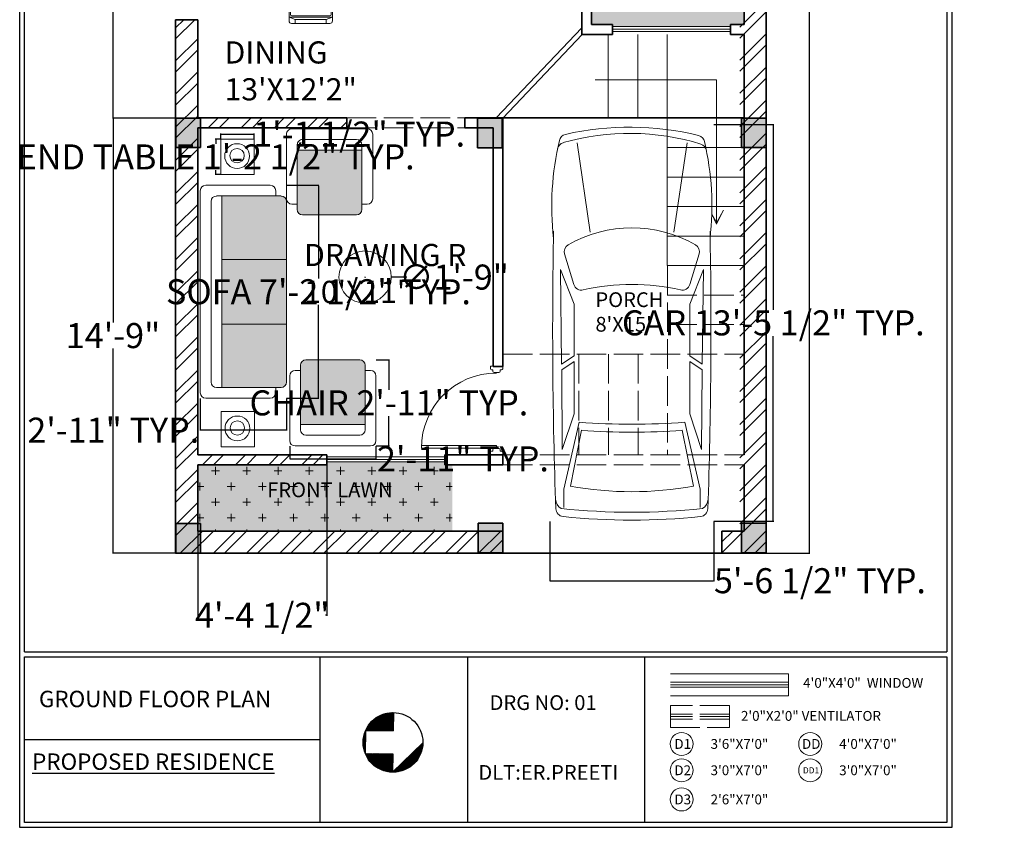
# Model space of a CAD drawing. Units: inches. Extents: x 1812 to 2791, y 2306 to 2959.
# Tile 5 of 8: x 2391 to 2791, y 2326 to 2655. Entities that reach past the tile are written whole.
import ezdxf

# ---------------------------------------------------------------- set-up
doc = ezdxf.new("R2010")
doc.units = ezdxf.units.IN
doc.linetypes.add('ACAD_ISO02W100', pattern=[15, 12, -3])
doc.layers.get('Defpoints').update_dxf_attribs({"lineweight": 50})
for name, color, linetype, lineweight in [('00 FURNITURE', 15, 'Continuous', 15), ('A-ANNO-DIMS', 2, 'Continuous', 18), ('A-ANNO-LEGD', 7, 'Continuous', 18), ('A-ANNO-SYMB', 7, 'Continuous', 18), ('A-ANNO-TEXT', 7, 'Continuous', 18), ('A-ANNO-TTLB', 7, 'Continuous', 25), ('A-AREA-IDEN', 7, 'Continuous', 18), ('A-COLS', 7, 'Continuous', 35), ('A-FLOR-STRS-OVHD', 30, 'ACAD_ISO02W100', 13), ('A-FURNITURE', 251, 'Continuous', 5), ('A-GLAZ-VENT', 6, 'ACAD_ISO02W100', 13), ('A-SITE-PARK', 8, 'Continuous', 13), ('A-WALL-OVHD', 30, 'ACAD_ISO02W100', 18), ('A-WALL-PATT', 8, 'Continuous', 13), ('DOORS', 4, 'Continuous', 18), ('L-PLNT-PATT', 8, 'Continuous', 13), ('STAIRCASE', 7, 'Continuous', 18), ('WALL', 7, 'Continuous', 35), ('WINDOWS', 160, 'Continuous', 18)]:
    doc.layers.add(name, color=color, linetype=linetype, lineweight=lineweight)
doc.layers.add('A-FURN-PATT', color=241, linetype='Continuous', lineweight=9, true_color=0xf7abae)
doc.layers.add('L-PLNT-TURF-PATT', color=116, linetype='Continuous', lineweight=9, true_color=0x136734)
doc.layers.add('WALLS', color=7, linetype='Continuous')
doc.styles.add('1-100DIM', font='txt', dxfattribs={"height": 0.3})
doc.styles.get("Standard").update_dxf_attribs({"font": 'arial.ttf'})
doc.dimstyles.get("Standard").update_dxf_attribs({"dimtxt": 10.18, "dimasz": 0.18, "dimexe": 0.18, "dimexo": 0.0625, "dimgap": 0.09, "dimtad": 0, "dimtih": 1, "dimtoh": 1, "dimdec": 0, "dimzin": 0, "dimdsep": 46, "dimlunit": 3, "dimtxsty": 'Standard', "dimcen": 0.09, "dimadec": 0, "dimazin": 0, "dimtfac": 1, "dimtdec": 0, "dimtofl": 0, "dimtmove": 0, "dimatfit": 3, "dimfxl": 1, "dimtolj": 1, "dimtzin": 0, "dimarcsym": 0})

# ---------------------------------------------------------------- blocks, each defined once
blk = doc.blocks.new('CAR')
at = {"layer": 'A-FURNITURE'}
for p, q in [((2677.91, 1665.57), (2683.24, 1629.33)), ((2722.63, 1665.57), (2717.3, 1629.33)), ((2672.85, 1620.44), (2676.61, 1608)), ((2727.48, 1620.44), (2723.73, 1608)), ((2671.15, 1614.07), (2676.73, 1600.01)), ((2671.63, 1575.61), (2671.15, 1614.07)), ((2729.25, 1614.07), (2723.67, 1600.01)), ((2728.77, 1575.61), (2729.25, 1614.07)), ((2676.73, 1600.01), (2676.73, 1578.97)), ((2723.67, 1600.01), (2723.67, 1578.97)), ((2676.73, 1578.97), (2671.63, 1575.61)), ((2676.73, 1576.71), (2671.66, 1573.38)), ((2676.73, 1576.71), (2676.73, 1555.46)), ((2723.67, 1578.97), (2728.77, 1575.61)), ((2723.67, 1576.71), (2723.67, 1555.46)), ((2723.67, 1576.71), (2728.74, 1573.38)), ((2671.9, 1540.91), (2671.66, 1573.38)), ((2728.49, 1540.91), (2728.74, 1573.38)), ((2676.73, 1555.46), (2671.9, 1540.91)), ((2723.67, 1555.46), (2728.49, 1540.91)), ((2678.77, 1552.01), (2672.52, 1524.85)), ((2675.22, 1526.01), (2679.74, 1548.74)), ((2725.17, 1526.01), (2720.66, 1548.74)), ((2721.71, 1552.02), (2727.96, 1524.85)), ((2672.52, 1524.85), (2672.52, 1517.39)), ((2727.96, 1524.85), (2727.96, 1517.39))]:
    blk.add_line(p, q, dxfattribs=at)
for centre, radius, start, end in [((2674, 1665.84), 3.34, 104.3452, 166.6607), ((2699.3, 1570.19), 99.28, 73.0347, 105.8141), ((2699.3, 1552.83), 119.14, 76.3976, 102.667), ((2726.43, 1665.41), 3.34, 13.1156, 74.5941), ((2783.1, 1639.97), 115.47, 166.6607, 186.5655), ((2673.27, 1662.52), 3.34, 107.8179, 168.3942), ((2727.17, 1661.99), 3.34, 11.3249, 70.8826), ((2617.23, 1639.97), 115.47, 353.4345, 13.1156), ((4741.11, 1589.62), 2073.11, 178.89024, 182.01225), ((2700.17, 1579.09), 51.94, 60.0774, 119.9226), ((659.22, 1589.62), 2073.11, 357.98775, 1.10976), ((2675.91, 1621.37), 3.2, 121.1455, 196.7984), ((2724.42, 1621.37), 3.2, 343.2016, 58.8545), ((2679.67, 1608.92), 3.2, 196.7984, 283.6631), ((2700.17, 1519.83), 88.22, 77.0683, 102.9317), ((2720.66, 1608.92), 3.2, 256.3369, 343.2016), ((2700.16, 1829.45), 278.26, 265.5919, 274.4407), ((2700.17, 1827.63), 279.65, 265.7971, 274.2029), ((2700.17, 1663.47), 139.72, 259.6897, 280.3103), ((2674.03, 1521.04), 4.9, 184.3987, 237.5288), ((2726.3, 1521.04), 4.9, 302.4712, 355.6013), ((2672.62, 1516.95), 3.34, 182.1119, 263.4899), ((2700.17, 1791.26), 275.86, 264.0142, 275.9858), ((2727.71, 1516.95), 3.34, 276.5101, 357.8881), ((2700.17, 1790.18), 277.96, 264.2342, 275.7658)]:
    blk.add_arc(centre, radius, start, end, dxfattribs=at)
blk = doc.blocks.new('CHAIR')
at = {"layer": '00 FURNITURE'}
for p, q in [((1778.29, 2628.74), (1800.19, 2628.74)), ((1776.1, 2600.27), (1776.1, 2626.55)), ((1802.38, 2626.55), (1802.38, 2600.27)), ((1771.72, 2595.89), (1771.72, 2622.17)), ((1773.91, 2624.36), (1776.1, 2624.36)), ((1802.38, 2624.36), (1804.57, 2624.36)), ((1806.76, 2622.17), (1806.76, 2595.89)), ((1802.38, 2602.46), (1776.1, 2602.46)), ((1800.19, 2598.08), (1778.29, 2598.08)), ((1804.57, 2593.7), (1773.91, 2593.7))]:
    blk.add_line(p, q, dxfattribs=at)
for centre, start, end in [((1778.29, 2626.55), 90, 180), ((1800.19, 2626.55), 0, 90), ((1773.91, 2622.17), 90, 180), ((1804.57, 2622.17), 0, 90), ((1778.29, 2600.27), 180, 270), ((1800.19, 2600.27), 270, 0), ((1773.91, 2595.89), 180, 270), ((1804.57, 2595.89), 270, 0)]:
    blk.add_arc(centre, 2.19, start, end, dxfattribs=at)
blk = doc.blocks.new('sofa 6')
for p, q in [((-1100, 167), (-1100, 834)), ((-1044, 890), (1044, 890)), ((1100, 834), (1100, 167)), ((-989, 56), (-989, 723)), ((-933, 779), (933, 779)), ((989, 723), (989, 56)), ((-989, 667), (989, 667)), ((-334, 667), (-334, 0)), ((334, 667), (334, 0)), ((-989, 111), (-1044, 111)), ((1044, 111), (989, 111)), ((933, 0), (-933, 0))]:
    blk.add_line(p, q)
for centre, start, end in [((-1044, 834), 90, 180), ((1044, 834), 0, 90), ((-933, 723), 90, 180), ((933, 723), 0, 90), ((-1044, 167), 180, 270), ((1044, 167), 270, 0), ((-933, 56), 180, 270), ((933, 56), 270, 0)]:
    blk.add_arc(centre, 55.6, start, end)
blk = doc.blocks.new('DDD')
at = {"layer": '00 FURNITURE'}
for p, q in [((-12579.77, -15859.53), (-12579.77, -15829.05)), ((-12578.77, -15859.53), (-12578.77, -15829.03)), ((-12612.02, -15857.03), (-12612.02, -15862.03)), ((-12611.02, -15857.03), (-12612.02, -15857.03)), ((-12610.52, -15858.03), (-12610.52, -15857.53)), ((-12577.52, -15858.03), (-12577.52, -15857.53)), ((-12577.02, -15857.03), (-12576.02, -15857.03)), ((-12576.02, -15857.03), (-12576.02, -15862.03)), ((-12612.02, -15862.03), (-12611.02, -15862.03)), ((-12610.52, -15861.53), (-12610.52, -15861.03)), ((-12578.77, -15859.53), (-12579.77, -15859.53)), ((-12577.52, -15861.53), (-12577.52, -15861.03)), ((-12576.02, -15862.03), (-12577.02, -15862.03))]:
    blk.add_line(p, q, dxfattribs=at)
for points in [[(-12610.52, -15861.03), (-12610.02, -15861.03, 0.414214), (-12609.52, -15860.53), (-12609.52, -15858.53, 0.414214), (-12610.02, -15858.03), (-12610.52, -15858.03)], [(-12577.52, -15861.03), (-12578.02, -15861.03, -0.414214), (-12578.52, -15860.53), (-12578.52, -15858.53, -0.414214), (-12578.02, -15858.03), (-12577.52, -15858.03)]]:
    blk.add_lwpolyline(points, format="xyb", dxfattribs=at)
for centre, radius, start, end in [((-12578.77, -15859.53), 30.5, 90, 180), ((-12611.02, -15857.53), 0.5, 0, 90), ((-12577.02, -15857.53), 0.5, 90, 180), ((-12611.02, -15861.53), 0.5, 270, 0), ((-12577.02, -15861.53), 0.5, 180, 270)]:
    blk.add_arc(centre, radius, start, end, dxfattribs=at)
blk = doc.blocks.new('*D25')
at = {"layer": 'A-ANNO-DIMS', "color": 0, "lineweight": -2, "transparency": 16777216}
for p, q in [((2694.21, 2918.01), (2711.94, 2918.01)), ((2711.76, 2917.83), (2711.76, 2683.09)), ((2711.76, 2437.78), (2711.76, 2672.52)), ((2694.21, 2437.6), (2711.94, 2437.6))]:
    blk.add_line(p, q, dxfattribs=at)
at = {"layer": 'A-ANNO-DIMS', "color": 0, "transparency": 16777216}
for points in [[(2711.73, 2917.83), (2711.79, 2917.83), (2711.76, 2918.01)], [(2711.73, 2437.78), (2711.79, 2437.78), (2711.76, 2437.6)]]:
    blk.add_solid(points, dxfattribs=at)
at = {"layer": 'Defpoints', "color": 0, "transparency": 16777216}
for p in [(2694.14, 2918.01), (2694.14, 2437.6), (2711.76, 2437.6)]:
    blk.add_point(p, dxfattribs=at)
at = {"layer": 'A-ANNO-DIMS', "color": 0, "transparency": 16777216, "insert": (2711.76, 2677.81), "char_height": 10.18, "attachment_point": 5}
blk.add_mtext("\\A1;40'", dxfattribs=at)
blk = doc.blocks.new('COL')
at = {"transparency": 33554687}
h = blk.add_hatch(color=256, dxfattribs=at)
h.dxf.hatch_style = 1
h.paths.add_polyline_path([(2424.4, 2829.24), (2424.4, 2839.24), (2412.4, 2839.24), (2412.4, 2829.24)])
for p, q in [((2412.4, 2839.24), (2424.4, 2839.24)), ((2412.4, 2839.24), (2412.4, 2829.24)), ((2424.4, 2839.24), (2424.4, 2829.24)), ((2412.4, 2829.24), (2424.4, 2829.24))]:
    blk.add_line(p, q)
blk = doc.blocks.new('NORTH')
at = {"layer": 'WALLS'}
h = blk.add_hatch(dxfattribs=at)
h.set_pattern_fill('ANSI31', color=256, scale=6.087211)
h.set_pattern_definition([(45, (-41048.0969, 128612.4242), (-0.53803848, 0.53803848), [])])
h.paths.add_polyline_path([(6704.42, -25696.22), (6687.22, -25696.22, 0.302843), (6704.42, -25722.01)])
h.paths.add_polyline_path([(6743.1, -25696.22), (6725.9, -25696.22), (6725.9, -25722.01, 0.302843)])
h.paths.add_polyline_path([(6715.16, -25668.28), (6743.1, -25696.22, 0.414214)])
h.paths.add_polyline_path([(6725.9, -25722.01), (6704.42, -25722.01, 0.199872)])
for p, q in [((6743.1, -25696.22, 0.29), (6715.16, -25668.28, 0.29)), ((6687.22, -25696.22, 0.29), (6704.42, -25696.22, 0.29)), ((6704.42, -25722.01, 0.29), (6704.42, -25696.22, 0.29)), ((6725.9, -25722.01, 0.29), (6725.9, -25696.22, 0.29)), ((6725.9, -25696.22, 0.29), (6743.1, -25696.22, 0.29)), ((6704.42, -25722.01, 0.29), (6725.9, -25722.01, 0.29))]:
    blk.add_line(p, q, dxfattribs=at)
blk.add_circle((6715.16, -25696.22, 0.29), 27.94, dxfattribs=at)
blk = doc.blocks.new('CHAIR-DINING')
for p, q in [((0, 16.64), (0, 1.02)), ((9.93, 17.65), (1.02, 17.65)), ((1.61, 15.13), (2.57, 17.65)), ((2.57, 17.65), (2.57, 0)), ((3.13, 16.53), (3.13, 1.12)), ((9.93, 17.09), (3.69, 17.09)), ((1.61, 15.13), (1.61, 2.55)), ((1.61, 2.55), (2.57, 0)), ((3.69, 0.56), (9.93, 0.56)), ((1.02, 0), (9.93, 0))]:
    blk.add_line(p, q)
blk.add_lwpolyline([(0, 15.13), (0, 2.55), (1.61, 2.55), (1.61, 15.13)], close=True)
for centre, radius, start, end in [((1.02, 16.64), 1.02, 89.9999, 179.9999), ((3.69, 16.53), 0.56, 89.9999, 179.9999), ((1.02, 1.02), 1.02, 179.9999, 269.9999), ((3.69, 1.12), 0.56, 179.9999, 269.9999)]:
    blk.add_arc(centre, radius, start, end)
blk = doc.blocks.new('TABLE-END-SQUARE')
blk.add_lwpolyline([(0, 14.29), (13.46, 14.29), (13.46, 0), (0, 0)], close=True)
for centre, radius in [((6.55, 7.48), 5.04), ((6.52, 7.65), 2.93)]:
    blk.add_circle(centre, radius)
blk = doc.blocks.new('VENT-24x9')
for p, q in [((3.5, 24), (3.5, 0)), ((4.5, 24), (4.5, 0)), ((5.5, 24), (5.5, 0))]:
    blk.add_line(p, q)
blk.add_lwpolyline([(0, 0), (9, 0), (9, 24), (0, 24)], close=True)
blk = doc.blocks.new('GLAZING-48x4')
for p, q in [((0, 2), (48, 2)), ((0, 1), (48, 1)), ((0, 0), (48, 0))]:
    blk.add_line(p, q)
blk = doc.blocks.new('WINDOW-LEGEND-48')
for p, q in [((48, 9), (0, 9)), ((48, 9), (48, 0)), ((48, 5.5), (0, 5.5)), ((48, 4.5), (0, 4.5)), ((48, 3.5), (0, 3.5)), ((0, 0), (48, 0))]:
    blk.add_line(p, q)
blk = doc.blocks.new('STAIR-DIRECTION')
for p, q in [((0, 58.78), (49.24, 58.78)), ((49.24, 58.78), (49.24, 0)), ((49.21, 0.29), (47.33, 4.04)), ((47.33, 4.04), (49.07, 1.3)), ((52.1, 5.77), (49.21, 0.29)), ((49.24, 0), (52.1, 5.77))]:
    blk.add_line(p, q)
blk = doc.blocks.new('SHEET-FRAME-RESIDENCE')
for p, q in [((2, 71.32), (376.76, 71.32)), ((2, 69.32), (376.76, 69.32)), ((122.05, 1.92), (122.05, 69.32)), ((182.05, 1.92), (182.05, 69.32)), ((254.05, 1.92), (254.05, 69.32)), ((2, 35.72), (122.05, 35.72))]:
    blk.add_line(p, q)
blk.add_lwpolyline([(0, 632.8), (378.76, 632.8), (378.76, 0), (0, 0)], close=True)
for points in [[(2, 71.32), (2, 630.8), (376.76, 630.8), (376.76, 71.32)], [(376.76, 69.32), (376.76, 2), (2, 2), (2, 69.32)]]:
    blk.add_lwpolyline(points)
blk = doc.blocks.new('*D40')
at = {"layer": 'A-ANNO-DIMS', "color": 0, "lineweight": -2, "transparency": 16777216}
for p, q in [((2535.66, 2516.27), (2541.04, 2516.27)), ((2540.86, 2516.09), (2540.86, 2504.11)), ((2540.86, 2481.42), (2540.86, 2493.4)), ((2535.66, 2481.24), (2541.04, 2481.24))]:
    blk.add_line(p, q, dxfattribs=at)
at = {"layer": 'A-ANNO-DIMS', "color": 0, "transparency": 16777216}
for points in [[(2540.83, 2516.09), (2540.89, 2516.09), (2540.86, 2516.27)], [(2540.83, 2481.42), (2540.89, 2481.42), (2540.86, 2481.24)]]:
    blk.add_solid(points, dxfattribs=at)
at = {"layer": 'Defpoints', "color": 0, "transparency": 16777216}
for p in [(2535.6, 2516.27), (2540.86, 2516.27), (2535.6, 2481.24)]:
    blk.add_point(p, dxfattribs=at)
at = {"layer": 'A-ANNO-DIMS', "color": 0, "transparency": 16777216, "insert": (2540.86, 2498.75), "char_height": 10.18, "attachment_point": 5}
blk.add_mtext('\\A1;CHAIR 2\'-11" TYP.', dxfattribs=at)
blk = doc.blocks.new('*D41')
at = {"layer": 'A-ANNO-DIMS', "color": 0, "lineweight": -2, "transparency": 16777216}
for p, q in [((2500.56, 2481.17), (2500.56, 2475.8)), ((2535.6, 2481.17), (2535.6, 2475.8)), ((2500.74, 2475.98), (2535.42, 2475.98)), ((2535.6, 2475.98), (2535.78, 2475.98))]:
    blk.add_line(p, q, dxfattribs=at)
at = {"layer": 'A-ANNO-DIMS', "color": 0, "transparency": 16777216}
for points in [[(2500.74, 2476.01), (2500.74, 2475.95), (2500.56, 2475.98)], [(2535.42, 2476.01), (2535.42, 2475.95), (2535.6, 2475.98)]]:
    blk.add_solid(points, dxfattribs=at)
at = {"layer": 'Defpoints', "color": 0, "transparency": 16777216}
for p in [(2500.56, 2481.24), (2535.6, 2481.24), (2535.6, 2475.98)]:
    blk.add_point(p, dxfattribs=at)
at = {"layer": 'A-ANNO-DIMS', "color": 0, "transparency": 16777216, "insert": (2570.94, 2475.98), "char_height": 10.18, "attachment_point": 5}
blk.add_mtext('\\A1;2\'-11" TYP.', dxfattribs=at)
blk = doc.blocks.new('*D44')
at = {"layer": 'A-ANNO-DIMS', "color": 0, "lineweight": -2, "transparency": 16777216}
for p, q in [((2472.56, 2605.93), (2470.3, 2605.93)), ((2470.48, 2605.75), (2470.48, 2604.14)), ((2470.48, 2591.82), (2470.48, 2593.43)), ((2472.56, 2591.64), (2470.3, 2591.64))]:
    blk.add_line(p, q, dxfattribs=at)
at = {"layer": 'A-ANNO-DIMS', "color": 0, "transparency": 16777216}
for points in [[(2470.45, 2605.75), (2470.51, 2605.75), (2470.48, 2605.93)], [(2470.45, 2591.82), (2470.51, 2591.82), (2470.48, 2591.64)]]:
    blk.add_solid(points, dxfattribs=at)
at = {"layer": 'Defpoints', "color": 0, "transparency": 16777216}
for p in [(2470.48, 2605.93), (2472.63, 2605.93), (2472.63, 2591.64)]:
    blk.add_point(p, dxfattribs=at)
at = {"layer": 'A-ANNO-DIMS', "color": 0, "transparency": 16777216, "insert": (2470.48, 2598.79), "char_height": 10.18, "attachment_point": 5}
blk.add_mtext('\\A1;END TABLE 1\'-2 1/2" TYP.', dxfattribs=at)
blk = doc.blocks.new('*D45')
at = {"layer": 'A-ANNO-DIMS', "color": 0, "lineweight": -2, "transparency": 16777216}
for p, q in [((2472.63, 2605.99), (2472.63, 2608.26)), ((2472.81, 2608.08), (2485.91, 2608.08)), ((2486.09, 2605.99), (2486.09, 2608.26)), ((2486.09, 2608.08), (2486.27, 2608.08))]:
    blk.add_line(p, q, dxfattribs=at)
at = {"layer": 'A-ANNO-DIMS', "color": 0, "transparency": 16777216}
for points in [[(2472.81, 2608.11), (2472.81, 2608.05), (2472.63, 2608.08)], [(2485.91, 2608.11), (2485.91, 2608.05), (2486.09, 2608.08)]]:
    blk.add_solid(points, dxfattribs=at)
at = {"layer": 'Defpoints', "color": 0, "transparency": 16777216}
for p in [(2472.63, 2605.93), (2486.09, 2608.08), (2486.09, 2605.93)]:
    blk.add_point(p, dxfattribs=at)
at = {"layer": 'A-ANNO-DIMS', "color": 0, "transparency": 16777216, "insert": (2528.77, 2608.08), "char_height": 10.18, "attachment_point": 5}
blk.add_mtext('\\A1;1\'-1 1/2" TYP.', dxfattribs=at)
blk = doc.blocks.new('*D52')
at = {"layer": 'A-ANNO-DIMS', "color": 0, "lineweight": -2, "transparency": 16777216}
for p, q in [((2672.92, 2611.96), (2697.23, 2611.96)), ((2697.05, 2611.78), (2697.05, 2536.65)), ((2697.05, 2450.81), (2697.05, 2525.93)), ((2672.92, 2450.63), (2697.23, 2450.63))]:
    blk.add_line(p, q, dxfattribs=at)
at = {"layer": 'A-ANNO-DIMS', "color": 0, "transparency": 16777216}
for points in [[(2697.02, 2611.78), (2697.08, 2611.78), (2697.05, 2611.96)], [(2697.02, 2450.81), (2697.08, 2450.81), (2697.05, 2450.63)]]:
    blk.add_solid(points, dxfattribs=at)
at = {"layer": 'Defpoints', "color": 0, "transparency": 16777216}
for p in [(2672.85, 2611.96), (2697.05, 2611.96), (2672.85, 2450.63)]:
    blk.add_point(p, dxfattribs=at)
at = {"layer": 'A-ANNO-DIMS', "color": 0, "transparency": 16777216, "insert": (2697.05, 2531.29), "char_height": 10.18, "attachment_point": 5}
blk.add_mtext('\\A1;CAR 13\'-5 1/2" TYP.', dxfattribs=at)
blk = doc.blocks.new('*D53')
at = {"layer": 'A-ANNO-DIMS', "color": 0, "lineweight": -2, "transparency": 16777216}
for p, q in [((2606.25, 2450.56), (2606.25, 2426.25)), ((2672.85, 2450.56), (2672.85, 2426.25)), ((2606.43, 2426.43), (2672.67, 2426.43)), ((2672.85, 2426.43), (2673.03, 2426.43))]:
    blk.add_line(p, q, dxfattribs=at)
at = {"layer": 'A-ANNO-DIMS', "color": 0, "transparency": 16777216}
for points in [[(2606.43, 2426.46), (2606.43, 2426.4), (2606.25, 2426.43)], [(2672.67, 2426.46), (2672.67, 2426.4), (2672.85, 2426.43)]]:
    blk.add_solid(points, dxfattribs=at)
at = {"layer": 'Defpoints', "color": 0, "transparency": 16777216}
for p in [(2606.25, 2450.63), (2672.85, 2450.63), (2672.85, 2426.43)]:
    blk.add_point(p, dxfattribs=at)
at = {"layer": 'A-ANNO-DIMS', "color": 0, "transparency": 16777216, "insert": (2716.01, 2426.43), "char_height": 10.18, "attachment_point": 5}
blk.add_mtext('\\A1;5\'-6 1/2" TYP.', dxfattribs=at)
blk = doc.blocks.new('*D54')
at = {"layer": 'A-ANNO-DIMS', "color": 0, "lineweight": -2, "transparency": 16777216}
for p, q in [((2499.3, 2587.25), (2512.41, 2587.25)), ((2512.23, 2587.07), (2512.23, 2549.3)), ((2512.23, 2500.82), (2512.23, 2538.59)), ((2499.3, 2500.64), (2512.41, 2500.64))]:
    blk.add_line(p, q, dxfattribs=at)
at = {"layer": 'A-ANNO-DIMS', "color": 0, "transparency": 16777216}
for points in [[(2512.2, 2587.07), (2512.26, 2587.07), (2512.23, 2587.25)], [(2512.2, 2500.82), (2512.26, 2500.82), (2512.23, 2500.64)]]:
    blk.add_solid(points, dxfattribs=at)
at = {"layer": 'Defpoints', "color": 0, "transparency": 16777216}
for p in [(2499.24, 2587.25), (2499.24, 2500.64), (2512.23, 2500.64)]:
    blk.add_point(p, dxfattribs=at)
at = {"layer": 'A-ANNO-DIMS', "color": 0, "transparency": 16777216, "insert": (2512.23, 2543.95), "char_height": 10.18, "attachment_point": 5}
blk.add_mtext('\\A1;SOFA 7\'-2 1/2" TYP.', dxfattribs=at)
blk = doc.blocks.new('*D55')
at = {"layer": 'A-ANNO-DIMS', "color": 0, "lineweight": -2, "transparency": 16777216}
for p, q in [((2464.2, 2500.58), (2464.2, 2487.47)), ((2499.24, 2500.58), (2499.24, 2487.47)), ((2464.2, 2487.65), (2464.02, 2487.65)), ((2499.06, 2487.65), (2464.38, 2487.65))]:
    blk.add_line(p, q, dxfattribs=at)
at = {"layer": 'A-ANNO-DIMS', "color": 0, "transparency": 16777216}
for points in [[(2464.38, 2487.68), (2464.38, 2487.62), (2464.2, 2487.65)], [(2499.06, 2487.68), (2499.06, 2487.62), (2499.24, 2487.65)]]:
    blk.add_solid(points, dxfattribs=at)
at = {"layer": 'Defpoints', "color": 0, "transparency": 16777216}
for p in [(2464.2, 2500.64), (2499.24, 2500.64), (2464.2, 2487.65)]:
    blk.add_point(p, dxfattribs=at)
at = {"layer": 'A-ANNO-DIMS', "color": 0, "transparency": 16777216, "insert": (2428.86, 2487.65), "char_height": 10.18, "attachment_point": 5}
blk.add_mtext('\\A1;2\'-11" TYP.', dxfattribs=at)
blk = doc.blocks.new('*D72')
at = {"layer": 'A-ANNO-DIMS', "color": 0, "lineweight": -2, "transparency": 16777216}
for p, q in [((2454.18, 2614.6), (2428.59, 2614.6)), ((2428.77, 2614.42), (2428.77, 2531.4)), ((2428.77, 2437.79), (2428.77, 2520.82)), ((2454.13, 2437.61), (2428.59, 2437.61))]:
    blk.add_line(p, q, dxfattribs=at)
at = {"layer": 'A-ANNO-DIMS', "color": 0, "transparency": 16777216}
for points in [[(2428.74, 2614.42), (2428.8, 2614.42), (2428.77, 2614.6)], [(2428.74, 2437.79), (2428.8, 2437.79), (2428.77, 2437.61)]]:
    blk.add_solid(points, dxfattribs=at)
at = {"layer": 'Defpoints', "color": 0, "transparency": 16777216}
for p in [(2428.77, 2614.6), (2454.24, 2614.6), (2454.19, 2437.61)]:
    blk.add_point(p, dxfattribs=at)
at = {"layer": 'A-ANNO-DIMS', "color": 0, "transparency": 16777216, "insert": (2428.77, 2526.11), "char_height": 10.18, "attachment_point": 5}
blk.add_mtext('\\A1;14\'-9"', dxfattribs=at)
blk = doc.blocks.new('*D73')
at = {"layer": 'A-ANNO-DIMS', "color": 0, "lineweight": -2, "transparency": 16777216}
for p, q in [((2454.22, 2760.69), (2428.59, 2760.69)), ((2428.77, 2760.51), (2428.77, 2692.85)), ((2428.77, 2614.78), (2428.77, 2682.45)), ((2454.18, 2614.6), (2428.59, 2614.6))]:
    blk.add_line(p, q, dxfattribs=at)
at = {"layer": 'A-ANNO-DIMS', "color": 0, "transparency": 16777216}
for points in [[(2428.74, 2760.51), (2428.8, 2760.51), (2428.77, 2760.69)], [(2428.74, 2614.78), (2428.8, 2614.78), (2428.77, 2614.6)]]:
    blk.add_solid(points, dxfattribs=at)
at = {"layer": 'Defpoints', "color": 0, "transparency": 16777216}
for p in [(2428.77, 2760.69), (2454.28, 2760.69), (2454.24, 2614.6)]:
    blk.add_point(p, dxfattribs=at)
at = {"layer": 'A-ANNO-DIMS', "color": 0, "transparency": 16777216, "insert": (2428.77, 2687.65), "char_height": 10.18, "attachment_point": 5}
blk.add_mtext('\\A1;12\'-2"', dxfattribs=at)
blk = doc.blocks.new('*D80')
at = {"layer": 'A-ANNO-DIMS', "color": 0, "lineweight": -2, "transparency": 16777216}
for p, q in [((2463.19, 2473.55), (2463.19, 2412.18)), ((2515.61, 2473.55), (2515.61, 2412.18)), ((2463.37, 2412.36), (2463.71, 2412.36)), ((2515.43, 2412.36), (2515.09, 2412.36))]:
    blk.add_line(p, q, dxfattribs=at)
at = {"layer": 'A-ANNO-DIMS', "color": 0, "transparency": 16777216}
for points in [[(2463.37, 2412.39), (2463.37, 2412.33), (2463.19, 2412.36)], [(2515.43, 2412.39), (2515.43, 2412.33), (2515.61, 2412.36)]]:
    blk.add_solid(points, dxfattribs=at)
at = {"layer": 'Defpoints', "color": 0, "transparency": 16777216}
for p in [(2463.19, 2473.61), (2515.61, 2473.61), (2515.61, 2412.36)]:
    blk.add_point(p, dxfattribs=at)
at = {"layer": 'A-ANNO-DIMS', "color": 0, "transparency": 16777216, "insert": (2489.4, 2412.36), "char_height": 10.18, "attachment_point": 5}
blk.add_mtext('\\A1;4\'-4 1/2"', dxfattribs=at)
blk = doc.blocks.new('*D88')
at = {"layer": 'A-ANNO-DIMS', "color": 0, "lineweight": -2, "transparency": 16777216}
for p, q in [((2531.11, 2549.91), (2531.29, 2549.91)), ((2531.2, 2549.82), (2531.2, 2550)), ((2548.2, 2549.91), (2542, 2549.91))]:
    blk.add_line(p, q, dxfattribs=at)
at = {"layer": 'A-ANNO-DIMS', "color": 0, "transparency": 16777216}
blk.add_solid([(2542, 2549.94), (2542, 2549.88), (2541.82, 2549.91)], dxfattribs=at)
at = {"layer": 'Defpoints', "color": 0, "transparency": 16777216}
for p in [(2520.58, 2549.91), (2541.82, 2549.91)]:
    blk.add_point(p, dxfattribs=at)
at = {"layer": 'A-ANNO-DIMS', "color": 0, "transparency": 16777216, "insert": (2567.35, 2549.91), "char_height": 10.18, "attachment_point": 5}
blk.add_mtext('\\A1;∅1\'-9"', dxfattribs=at)

msp = doc.modelspace()

# ---------------------------------------------------------------- hatches: boundary and pattern name
at = {"layer": 'A-FURN-PATT', "transparency": 33554534}
h = msp.add_hatch(color=256, dxfattribs=at)
h.dxf.hatch_style = 1
h.paths.add_polyline_path([(2685.19, 2760.61), (2617.42, 2760.61), (2617.42, 2736.61), (2661.19, 2736.61), (2661.19, 2676.61), (2623.19, 2676.61), (2623.19, 2652.61), (2631.67, 2652.61), (2631.67, 2651.78), (2679.67, 2651.78), (2679.67, 2652.61), (2685.19, 2652.61)])
h.paths.add_polyline_path([(2664.17, 2733.97), (2682.07, 2733.97), (2682.07, 2702.86), (2664.17, 2702.86), (2664.17, 2704.82), (2663.38, 2704.82), (2663.38, 2731.7), (2664.17, 2731.7)], flags=16)
h.paths.add_polyline_path([(2675.01, 2727.15, -1), (2668.73, 2727.15, -1)], flags=0)
h.paths.add_polyline_path([(2675.4, 2710.4, -1), (2668.34, 2710.4, -1)], flags=0)
h.paths.add_polyline_path([(2685.16, 2788.57), (2576.48, 2788.57), (2576.48, 2764.61), (2685.16, 2764.61)])
h.paths.add_polyline_path([(2617.42, 2760.61), (2575.19, 2760.61), (2575.19, 2736.61), (2617.42, 2736.61)])
h.paths.add_polyline_path([(2499.24, 2557.09), (2472.96, 2557.09), (2472.96, 2530.81), (2499.24, 2530.81)])
h.paths.add_polyline_path([(2499.24, 2580.68, 0.414214), (2497.05, 2582.87), (2472.96, 2582.87), (2472.96, 2557.09), (2499.24, 2557.09)])
h.paths.add_polyline_path([(2529.89, 2601.46), (2503.61, 2601.46), (2503.61, 2577.37, 0.414214), (2505.8, 2575.18), (2527.7, 2575.18, 0.414214), (2529.89, 2577.37)])
h.paths.add_polyline_path([(2499.24, 2530.81), (2472.96, 2530.81), (2472.96, 2505.02), (2497.05, 2505.02, 0.414214), (2499.24, 2507.21)])
h.paths.add_polyline_path([(2531.22, 2514.08, 0.414214), (2529.03, 2516.27), (2507.13, 2516.27, 0.414214), (2504.94, 2514.08), (2504.94, 2489.99), (2531.22, 2489.99)])
h.paths.add_polyline_path([(2613.92, 2898.81, 0.308459), (2611.87, 2898.95, 0.065472), (2601.84, 2888.94), (2601.74, 2888.94, 0.386143), (2601.79, 2886.97, 0.011497), (2611.24, 2877.54, 0.265248), (2613.05, 2877.56, 0.066056), (2623.16, 2887.66, 0.308904), (2623.02, 2889.71, 0.059418)])
h.paths.add_polyline_path([(2624.7, 2898.81, 0.308459), (2622.65, 2898.95, 0.027227), (2618.16, 2895.1, -0.033416), (2623.02, 2889.72, -0.379362), (2622.88, 2887.3, -0.036525), (2617.56, 2881.42, 0.027343), (2622.04, 2877.53, 0.262295), (2623.83, 2877.56, 0.066056), (2633.94, 2887.66, 0.308904), (2633.8, 2889.71, 0.059418)])
h.paths.add_polyline_path([(2656.38, 2844.47), (2643.48, 2831.57), (2655.48, 2831.57, 0.414214), (2656.38, 2832.47)], flags=17)
h.paths.add_polyline_path([(2656.38, 2880.07), (2655.64, 2880.07, 0.052719), (2600.4, 2868.59, 0.295777), (2591.58, 2880.13), (2591.58, 2832.47, 0.414214), (2592.48, 2831.57), (2614.43, 2831.57), (2643.48, 2831.57, 0.253465), (2646.43, 2841.52, 0.253465), (2656.38, 2844.47)])
h.paths.add_polyline_path([(2655.64, 2880.07), (2626.88, 2880.07, -0.016036), (2624.2, 2877.84, -0.429576), (2621.56, 2877.91, -0.015371), (2619.01, 2880.07), (2616.1, 2880.07, -0.016036), (2613.42, 2877.84, -0.334836), (2611.24, 2877.54, -0.003141), (2608.62, 2880.07), (2591.75, 2880.07, -0.292232), (2600.4, 2868.59, -0.052719)], flags=17)
h.paths.add_polyline_path([(2656.39, 2844.48, -0.2538), (2646.43, 2841.52, -0.253465), (2643.48, 2831.57)])
h.paths.add_polyline_path([(2656.38, 2907.17), (2591.58, 2907.17), (2591.58, 2903.52), (2656.38, 2903.52)])
at = {"layer": 'A-WALL-PATT'}
h = msp.add_hatch(dxfattribs=at)
h.set_pattern_fill('ANSI32', color=256)
h.set_pattern_definition([(45, (563.806, 20.011), (-6.735192, 6.735192), []), (45, (568.296, 20.011), (-6.735192, 6.735192), [])])
h.paths.add_polyline_path([(2694.19, 2437.61), (2683.5, 2437.61), (2683.5, 2788.57), (2685.19, 2788.57), (2685.19, 2821.64), (2685.13, 2869.37), (2685.13, 2821.64), (2694.19, 2821.64)])
h.paths.add_polyline_path([(2587.19, 2446.61), (2463.19, 2446.61), (2463.19, 2473.61), (2515.61, 2473.61), (2515.61, 2477.61), (2463.19, 2477.61), (2463.19, 2610.61), (2523.74, 2610.61), (2523.74, 2614.61), (2463.19, 2614.61), (2463.19, 2654.54), (2454.19, 2654.54), (2454.19, 2437.61), (2587.19, 2437.61)])
h.paths.add_polyline_path([(2683.5, 2446.61), (2676.19, 2446.61), (2676.19, 2437.61), (2683.5, 2437.61)])
h.paths.add_polyline_path([(2463.19, 2760.61), (2505.19, 2760.61), (2505.19, 2764.61), (2463.19, 2764.61), (2463.19, 2792.95), (2454.19, 2792.95), (2454.19, 2702.54), (2463.02, 2702.54), (2463.02, 2702.65)])
h.paths.add_polyline_path([(2539.19, 2858.61), (2463.19, 2858.61), (2463.19, 2876.35), (2454.19, 2876.35), (2454.19, 2816.96), (2463.19, 2816.96), (2463.19, 2854.61), (2535.19, 2854.61), (2535.19, 2760.61), (2539.19, 2760.61)])
h.paths.add_polyline_path([(2683.5, 2917.61), (2454.19, 2917.61), (2454.19, 2900.37), (2463.19, 2900.37), (2463.19, 2908.61), (2683.5, 2908.61)])
h.paths.add_polyline_path([(2694.19, 2917.61), (2683.5, 2917.61), (2683.5, 2908.61), (2685.19, 2908.61), (2685.19, 2869.64), (2694.19, 2869.64)])
at = {"layer": 'L-PLNT-PATT'}
h = msp.add_hatch(dxfattribs=at)
h.set_pattern_fill('CROSS', color=256)
h.set_pattern_definition([(0, (563.806, 20.0107), (6.35, 6.35), [3.175, -9.525]), (90, (565.393, 18.423), (-6.35, 6.35), [3.175, -9.525])])
h.paths.add_polyline_path([(2566.63, 2473.61), (2563.61, 2473.61), (2563.61, 2474.75), (2515.61, 2474.75), (2515.61, 2473.61), (2463.19, 2473.61), (2463.19, 2446.61), (2566.63, 2446.61)])
h.paths.add_polyline_path([(2489.21, 2457.01), (2547.62, 2457.01), (2547.62, 2469.38), (2489.21, 2469.38)], flags=24)
at = {"layer": 'L-PLNT-TURF-PATT', "transparency": 33554585}
h = msp.add_hatch(color=256, dxfattribs=at)
h.dxf.hatch_style = 1
h.paths.add_polyline_path([(2566.63, 2473.61), (2563.61, 2473.61), (2563.61, 2474.75), (2515.61, 2474.75), (2515.61, 2473.61), (2463.19, 2473.61), (2463.19, 2446.61), (2566.63, 2446.61)])
h.paths.add_polyline_path([(2489.21, 2457.01), (2547.62, 2457.01), (2547.62, 2469.38), (2489.21, 2469.38)], flags=24)

# ---------------------------------------------------------------- linework, layer by layer
at = {"layer": '00 FURNITURE'}
msp.add_circle((2531.2, 2549.91), 10.62, dxfattribs=at)
at = {"layer": 'A-ANNO-LEGD'}
for centre in [(2659.79, 2360.04), (2712.04, 2360.04), (2659.79, 2349.32), (2712.04, 2349.32), (2659.79, 2337.47)]:
    msp.add_circle(centre, 4.67, dxfattribs=at)
at = {"layer": 'A-FLOR-STRS-OVHD'}
for p, q in [((2654.09, 2554.61), (2654.09, 2477.61)), ((2653.99, 2542.61), (2685.19, 2542.61)), ((2653.99, 2530.61), (2685.19, 2530.61)), ((2587.19, 2518.61), (2685.19, 2518.61)), ((2618.09, 2518.61), (2618.09, 2477.61)), ((2630.09, 2518.61), (2630.09, 2477.61)), ((2642.09, 2518.61), (2642.09, 2477.61))]:
    msp.add_line(p, q, dxfattribs=at)
at = {"layer": 'A-WALL-OVHD'}
for p, q in [((2523.74, 2614.61), (2571.74, 2614.61)), ((2523.74, 2610.61), (2571.74, 2610.61)), ((2587.19, 2477.61), (2685.19, 2477.61)), ((2587.19, 2473.61), (2685.19, 2473.61))]:
    msp.add_line(p, q, dxfattribs=at)
at = {"layer": 'STAIRCASE'}
for p, q in [((2629.99, 2648.61), (2629.99, 2614.61)), ((2641.99, 2648.61), (2641.99, 2614.61)), ((2653.99, 2648.61), (2653.99, 2554.61)), ((2653.99, 2602.61), (2685.19, 2602.61)), ((2653.99, 2590.61), (2685.19, 2590.61)), ((2653.99, 2578.61), (2685.19, 2578.61)), ((2653.99, 2566.61), (2685.19, 2566.61)), ((2653.99, 2554.61), (2685.19, 2554.61))]:
    msp.add_line(p, q, dxfattribs=at)
at = {"layer": 'WALL'}
for p, q in [((2694.19, 2821.64), (2694.19, 2437.61)), ((2685.19, 2760.61), (2685.19, 2652.61)), ((2619.19, 2648.61), (2619.19, 2676.61)), ((2623.19, 2652.61), (2623.19, 2676.61)), ((2454.19, 2437.61), (2454.19, 2654.54)), ((2454.19, 2654.54), (2463.19, 2654.54)), ((2463.19, 2614.61), (2463.19, 2654.54)), ((2623.19, 2652.61), (2631.67, 2652.61)), ((2631.67, 2648.61), (2631.67, 2652.61)), ((2679.67, 2652.61), (2685.19, 2652.61)), ((2679.67, 2648.61), (2679.67, 2652.61)), ((2584.5, 2614.61), (2619.19, 2651.29)), ((2587.19, 2614.55), (2619.41, 2648.61)), ((2619.19, 2648.61), (2631.67, 2648.61)), ((2679.67, 2648.61), (2685.19, 2648.61)), ((2685.19, 2648.61), (2685.19, 2477.61)), ((2463.19, 2614.61), (2523.74, 2614.61)), ((2523.74, 2610.61), (2523.74, 2614.61)), ((2571.74, 2614.61), (2685.19, 2614.61)), ((2571.74, 2610.61), (2571.74, 2614.61)), ((2587.19, 2513.61), (2587.19, 2614.61)), ((2463.19, 2610.61), (2523.74, 2610.61)), ((2463.19, 2477.61), (2463.19, 2610.61)), ((2571.74, 2610.61), (2583.19, 2610.61)), ((2583.19, 2513.61), (2583.19, 2610.61)), ((2587.19, 2513.61), (2583.19, 2513.61)), ((2515.61, 2477.61), (2463.19, 2477.61)), ((2515.61, 2473.61), (2515.61, 2477.61)), ((2587.19, 2477.61), (2563.61, 2477.61)), ((2563.61, 2473.61), (2563.61, 2477.61)), ((2587.19, 2473.61), (2587.19, 2477.61)), ((2515.61, 2473.61), (2463.19, 2473.61)), ((2463.19, 2446.61), (2463.19, 2473.61)), ((2587.19, 2473.61), (2563.61, 2473.61)), ((2685.19, 2473.61), (2685.19, 2446.61)), ((2587.19, 2446.61), (2463.19, 2446.61)), ((2587.19, 2437.61), (2587.19, 2446.61)), ((2676.19, 2446.61), (2676.19, 2437.61)), ((2685.19, 2446.61), (2676.19, 2446.61)), ((2676.19, 2437.61), (2454.19, 2437.61)), ((2694.19, 2437.61), (2676.19, 2437.61))]:
    msp.add_line(p, q, dxfattribs=at)
at = {"layer": 'WINDOWS'}
for p, q in [((2679.54, 2651.78), (2631.54, 2651.78)), ((2679.54, 2650.78), (2631.54, 2650.78)), ((2679.54, 2649.78), (2631.54, 2649.78))]:
    msp.add_line(p, q, dxfattribs=at)

# ---------------------------------------------------------------- block references
at = {"layer": '00 FURNITURE', "extrusion": (0, 0, -1), "zscale": -1, "rotation": 90.00000000029095}
msp.add_blockref('CHAIR-DINING', (-2500.27, 2653.06), dxfattribs=at)
at = {"layer": '00 FURNITURE', "rotation": 180}
msp.add_blockref('CHAIR', (4305.99, 5203.92), dxfattribs=at)
at = {"layer": '00 FURNITURE'}
for name, p in [('TABLE-END-SQUARE', (2472.63, 2591.64)), ('CHAIR', (728.84, -112.47)), ('TABLE-END-SQUARE', (2472.75, 2480.89))]:
    msp.add_blockref(name, p, dxfattribs=at)
at = {"layer": '00 FURNITURE', "xscale": -0.0393700787401575, "yscale": 0.0393700787401575, "zscale": 0.0393700787401575, "rotation": 90}
msp.add_blockref('sofa 6', (2499.24, 2543.95), dxfattribs=at)
at = {"layer": 'A-ANNO-LEGD'}
msp.add_blockref('WINDOW-LEGEND-48', (2655.22, 2379.62), dxfattribs=at)
at = {"layer": 'A-ANNO-SYMB'}
msp.add_blockref('STAIR-DIRECTION', (2624.68, 2571.4), dxfattribs=at)
at = {"layer": 'A-ANNO-SYMB', "xscale": 0.4341621291417894, "yscale": 0.4341621291417894, "zscale": 0.4341621291417894, "rotation": 269.2509902977627}
msp.add_blockref('NORTH', (13736, 5130.06, -0.13), dxfattribs=at)
at = {"layer": 'A-ANNO-TTLB'}
msp.add_blockref('SHEET-FRAME-RESIDENCE', (2390.83, 2326.13), dxfattribs=at)
at = {"layer": 'A-COLS', "rotation": 270}
for p in [(-375, 5027), (-252.33, 5026.92), (-145.05, 5026.99), (-374.99, 4862.06), (-252.12, 4862.19), (-145.14, 4862.19)]:
    msp.add_blockref('COL', p, dxfattribs=at)
at = {"layer": 'A-GLAZ-VENT', "rotation": 269.9999999999993}
msp.add_blockref('VENT-24x9', (2655.22, 2375.67), dxfattribs=at)
at = {"layer": 'A-SITE-PARK'}
msp.add_blockref('CAR', (-60.6, 938.87), dxfattribs=at)
at = {"layer": 'DOORS', "xscale": -1, "rotation": 90}
msp.add_blockref('DDD', (-13274.94, -10098.38), dxfattribs=at)
at = {"layer": 'WINDOWS', "rotation": 180}
msp.add_blockref('GLAZING-48x4', (2563.62, 2476.75), dxfattribs=at)

# ---------------------------------------------------------------- texts
at = {"layer": 'A-ANNO-TEXT', "attachment_point": 1}
for s, width, insert, char_height in [('4\'0"X4\'0"  WINDOW', 55.3456, (2709.16, 2386.87), 4), ('2\'0"X2\'0" VENTILATOR', 67.3186, (2683.91, 2373.45), 4), ('D1', 8.4888, (2656.85, 2362.05), 4), ('3\'6"X7\'0"', 8.4888, (2671.57, 2362.05), 4), ('DD', 8.4888, (2708.69, 2362.05), 4), ('4\'0"X7\'0"', 8.4888, (2723.82, 2362.05), 4), ('D2', 8.4888, (2656.85, 2351.34), 4), ('3\'0"X7\'0"', 8.4888, (2671.57, 2351.34), 4), ('DD1', 8.4888, (2709.1, 2350.56), 2.5), ('3\'0"X7\'0"', 8.4888, (2723.82, 2351.34), 4), ('D3', 8.4888, (2656.85, 2339.48), 4), ('2\'6"X7\'0"', 8.4888, (2671.57, 2339.48), 4)]:
    msp.add_mtext_dynamic_manual_height_columns(s, width=width, gutter_width=12.5, heights=[0], dxfattribs=dict(at, insert=insert, char_height=char_height))
at = {"layer": 'A-ANNO-TTLB', "char_height": 6.6726, "attachment_point": 1, "style": '1-100DIM'}
for s, width, insert in [('{\\f@Malgun Gothic|b0|i0|c0|p34;GROUND FLOOR PLAN }', 159.0041, (2398.65, 2381.67)), ('{\\f@Malgun Gothic|b0|i0|c0|p34;\\LPROPOSED RESIDENCE   }', 252.3616, (2395.9, 2356.18))]:
    msp.add_mtext_dynamic_manual_height_columns(s, width=width, gutter_width=13.96, heights=[0], dxfattribs=dict(at, insert=insert))
at = {"layer": 'A-ANNO-TTLB', "char_height": 6, "attachment_point": 1}
for s, insert in [('DRG NO: 01', (2581.77, 2379.85)), ('\\PDLT:ER.PREETI', (2577.21, 2361.48))]:
    msp.add_mtext_dynamic_manual_height_columns(s, width=58.1461, gutter_width=12.5, heights=[0], dxfattribs=dict(at, insert=insert))
at = {"layer": 'A-AREA-IDEN', "attachment_point": 1}
for s, width, insert, char_height in [('DINING\\P13\'X12\'2"', 96.4869, (2474.08, 2645.77), 9), ("DRAWING R\\P10'X11'", 96.4869, (2506.38, 2563.39), 9), ("PORCH\\P8'X15'", 184.4395, (2624.78, 2543.72), 6), ('FRONT LAWN', 184.4395, (2491.4, 2466.39), 6)]:
    msp.add_mtext_dynamic_manual_height_columns(s, width=width, gutter_width=12.5, heights=[0], dxfattribs=dict(at, insert=insert, char_height=char_height))

# ---------------------------------------------------------------- dimensions: what is measured, and where the dimension line sits
at = {"layer": 'A-ANNO-DIMS'}
dim = msp.add_linear_dim(base=(2711.76, 2437.6), p1=(2694.14, 2918.01), p2=(2694.14, 2437.6), angle=90, dimstyle='Standard', override={"dimclrd": 0, "dimclre": 0, "dimclrt": 0}, dxfattribs=at)
dim.commit()
dim.dimension.update_dxf_attribs({"geometry": '*D25', "text_midpoint": (2711.76, 2677.81), "dimtype": 160})
for base, p1, p2, picture, middle in [((2428.77, 2760.69), (2454.24, 2614.6), (2454.28, 2760.69), '*D73', (2428.77, 2687.65)), ((2428.77, 2614.6), (2454.19, 2437.61), (2454.24, 2614.6), '*D72', (2428.77, 2526.11))]:
    dim = msp.add_linear_dim(base=base, p1=p1, p2=p2, angle=90, dimstyle='Standard', override={"dimdec": 1, "dimlfac": 1, "dimrnd": 0, "dimzin": 1, "dimdsep": 46, "dimlunit": 4, "dimfrac": 2}, dxfattribs=at)
    dim.commit()
    dim.dimension.update_dxf_attribs({"geometry": picture, "text_midpoint": middle})
for base, p1, p2, angle, text, picture, middle in [((2470.48, 2605.93), (2472.63, 2591.64), (2472.63, 2605.93), 90, 'END TABLE <> TYP.', '*D44', (2470.48, 2598.79)), ((2697.05, 2611.96), (2672.85, 2450.63), (2672.85, 2611.96), 90, 'CAR <> TYP.', '*D52', (2697.05, 2531.29)), ((2512.23, 2500.64), (2499.24, 2587.25), (2499.24, 2500.64), 270, 'SOFA <> TYP.', '*D54', (2512.23, 2543.95)), ((2540.86, 2516.27), (2535.6, 2481.24), (2535.6, 2516.27), 90, 'CHAIR <> TYP.', '*D40', (2540.86, 2498.75)), ((2464.2, 2487.65), (2499.24, 2500.64), (2464.2, 2500.64), 180, '<> TYP.', '*D55', (2428.86, 2487.65))]:
    dim = msp.add_linear_dim(base=base, p1=p1, p2=p2, angle=angle, text=text, dimstyle='Standard', override={"dimdec": 1, "dimlfac": 1, "dimrnd": 0, "dimzin": 1, "dimdsep": 46, "dimlunit": 4, "dimfrac": 2}, dxfattribs=at)
    dim.commit()
    dim.dimension.update_dxf_attribs({"geometry": picture, "text_midpoint": middle})
for base, p1, p2, picture, middle in [((2486.09, 2608.08), (2472.63, 2605.93), (2486.09, 2605.93), '*D45', (2528.77, 2608.08)), ((2535.6, 2475.98), (2500.56, 2481.24), (2535.6, 2481.24), '*D41', (2570.94, 2475.98)), ((2672.85, 2426.43), (2606.25, 2450.63), (2672.85, 2450.63), '*D53', (2716.01, 2426.43))]:
    dim = msp.add_linear_dim(base=base, p1=p1, p2=p2, text='<> TYP.', dimstyle='Standard', override={"dimdec": 1, "dimlfac": 1, "dimrnd": 0, "dimzin": 1, "dimdsep": 46, "dimlunit": 4, "dimfrac": 2}, dxfattribs=at)
    dim.commit()
    dim.dimension.update_dxf_attribs({"geometry": picture, "text_midpoint": middle})
dim = msp.add_diameter_dim_2p(p1=(2520.58, 2549.91), p2=(2541.82, 2549.91), dimstyle='Standard', override={"dimdec": 1, "dimlfac": 1, "dimrnd": 0, "dimzin": 1, "dimdsep": 46, "dimlunit": 4, "dimfrac": 2}, dxfattribs=at)
dim.commit()
dim.dimension.update_dxf_attribs({"geometry": '*D88', "text_midpoint": (2548.2, 2549.91), "dimtype": 163})
dim = msp.add_linear_dim(base=(2515.61, 2412.36), p1=(2463.19, 2473.61), p2=(2515.61, 2473.61), dimstyle='Standard', override={"dimdec": 1, "dimlfac": 1, "dimrnd": 0, "dimzin": 1, "dimdsep": 46, "dimlunit": 4, "dimfrac": 2}, dxfattribs=at)
dim.commit()
dim.dimension.update_dxf_attribs({"geometry": '*D80', "text_midpoint": (2489.4, 2412.36)})

doc.saveas('drawing.dxf')
